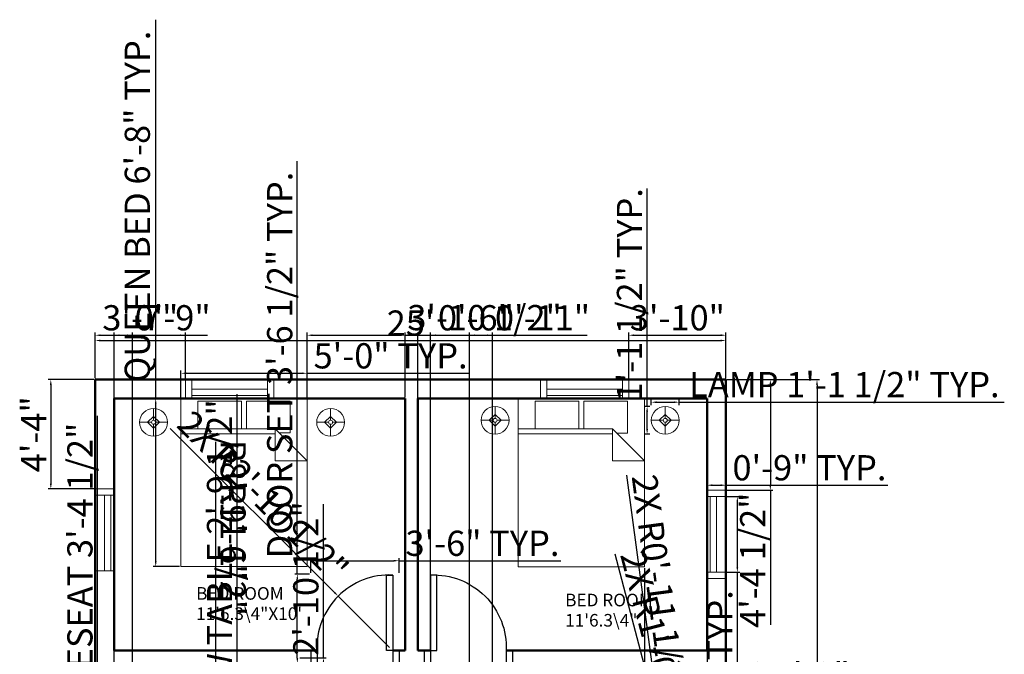
# Model space of a CAD drawing. Units: inches. Extents: x 3705 to 4206, y -1241 to -584.
# Tile 3 of 3: x 3738 to 4206, y -886 to -584. Entities that reach past the tile are written whole.
import ezdxf

# ---------------------------------------------------------------- set-up
doc = ezdxf.new("R2010")
doc.units = ezdxf.units.IN
for name, color, linetype, lineweight in [('A-ANNO-DIMS', 2, 'Continuous', 18), ('A-AREA-IDEN', 7, 'Continuous', 25), ('A-DOOR', 3, 'Continuous', 25), ('A-FURN', 8, 'Continuous', 18), ('A-GLAZ', 4, 'Continuous', 18), ('A-WALL', 7, 'Continuous', 50)]:
    doc.layers.add(name, color=color, linetype=linetype, lineweight=lineweight)
doc.styles.get("Standard").update_dxf_attribs({"font": 'arial.ttf'})
doc.dimstyles.new('ISO-25', dxfattribs={"dimtxt": 12, "dimasz": 2.5, "dimexe": 1.25, "dimexo": 0.625, "dimtad": 1, "dimdec": 1, "dimlunit": 3, "dimtxsty": 'Standard', "dimcen": 2.5, "dimadec": 0, "dimazin": 0, "dimtfac": 1, "dimtdec": 1, "dimtmove": 0, "dimatfit": 3, "dimfxl": 1, "dimarcsym": 0})

# ---------------------------------------------------------------- blocks, each defined once
blk = doc.blocks.new('Bed - Queen')
for p, q in [((0, -80.00003), (0, 0)), ((0, 0), (59.99999, 0)), ((59.99999, 0), (59.99999, -80.00003)), ((7.99999, -1.2), (28.79998, -1.2)), ((7.99999, -14.4), (7.99999, -1.2)), ((28.79998, -1.2), (28.79998, -14.4)), ((31.19999, -1.2), (51.99999, -1.2)), ((31.19999, -14.4), (31.19999, -1.2)), ((51.99999, -1.2), (51.99999, -16.4)), ((0, -14.4), (44.8, -14.4)), ((44.8, -16.8), (0, -16.8)), ((59.99999, -29.6), (44.8, -14.4)), ((44.8, -14.4), (44.8, -29.6)), ((51.99999, -16.4), (46.79936, -16.4)), ((44.8, -29.6), (59.99999, -29.6)), ((59.99999, -80.00003), (0, -80.00003))]:
    blk.add_line(p, q)
blk = doc.blocks.new('Lamp - Table')
for p, q in [((0, 7), (0, 1)), ((-1, 0), (-7, 0)), ((0, 3), (-3, 0)), ((-3, 0), (0, -3)), ((3, 0), (0, 3)), ((0, -3), (3, 0)), ((1, 0), (7, 0)), ((0, -1), (0, -7))]:
    blk.add_line(p, q)
for radius in [7, 1]:
    blk.add_circle((0, 0), radius)
blk = doc.blocks.new('*D11')
at = {"layer": 'A-ANNO-DIMS', "color": 0, "lineweight": -2, "transparency": 16777216}
for p, q in [((3774.08, -755.12), (3774.08, -735.92)), ((3776.58, -737.17), (4071.58, -737.17)), ((4074.08, -755.12), (4074.08, -735.92))]:
    blk.add_line(p, q, dxfattribs=at)
at = {"layer": 'A-ANNO-DIMS', "color": 0, "transparency": 16777216}
for points in [[(3776.58, -736.75), (3776.58, -737.58), (3774.08, -737.17)], [(4071.58, -736.75), (4071.58, -737.58), (4074.08, -737.17)]]:
    blk.add_solid(points, dxfattribs=at)
at = {"layer": 'Defpoints', "color": 0, "transparency": 16777216}
for p in [(4074.08, -737.17), (3774.08, -755.75), (4074.08, -755.75)]:
    blk.add_point(p, dxfattribs=at)
at = {"layer": 'A-ANNO-DIMS', "color": 0, "transparency": 16777216, "insert": (3924.08, -730.42), "char_height": 12, "attachment_point": 5}
blk.add_mtext("25'", dxfattribs=at)
blk = doc.blocks.new('*D12')
at = {"layer": 'A-ANNO-DIMS', "color": 0, "lineweight": -2, "transparency": 16777216}
for p, q in [((4074.7, -755.75), (4118.62, -755.75)), ((4117.37, -758.25), (4117.37, -1137.25)), ((4074.7, -1139.75), (4118.62, -1139.75))]:
    blk.add_line(p, q, dxfattribs=at)
at = {"layer": 'A-ANNO-DIMS', "color": 0, "transparency": 16777216}
for points in [[(4116.95, -758.25), (4117.78, -758.25), (4117.37, -755.75)], [(4116.95, -1137.25), (4117.78, -1137.25), (4117.37, -1139.75)]]:
    blk.add_solid(points, dxfattribs=at)
at = {"layer": 'Defpoints', "color": 0, "transparency": 16777216}
for p in [(4074.08, -755.75), (4074.08, -1139.75), (4117.37, -1139.75)]:
    blk.add_point(p, dxfattribs=at)
at = {"layer": 'A-ANNO-DIMS', "color": 0, "transparency": 16777216, "insert": (4110.61, -947.75), "char_height": 12, "attachment_point": 5, "rotation": 90}
blk.add_mtext("32'", dxfattribs=at)
blk = doc.blocks.new('DOOR-SINGLE-36IN')
for p, q in [((0, 6), (0, 0)), ((3, 6), (3, 0)), ((39, 6), (39, 0)), ((42, 6), (42, 0))]:
    blk.add_line(p, q)
blk.add_lwpolyline([(39, 6), (36, 6), (36, 42), (39, 42)], close=True)
blk.add_arc((37.5, 7.5), 34.53, 87.5104, 182.4896)
blk = doc.blocks.new('WIN-SASH-36IN')
for p, q in [((0, 9), (0, 0)), ((36, 0), (36, 9)), ((0, 4.5), (36, 4.5)), ((0, 1.5), (36, 1.5)), ((0, 1.5), (36, 1.5))]:
    blk.add_line(p, q)
blk = doc.blocks.new('*D15')
at = {"layer": 'A-ANNO-DIMS', "color": 0, "lineweight": -2, "transparency": 16777216}
for p, q in [((4074.7, -811.42), (4080.73, -811.42)), ((4079.48, -813.92), (4079.48, -844.92)), ((4074.7, -847.42), (4080.73, -847.42)), ((4079.48, -847.42), (4079.48, -1052.78))]:
    blk.add_line(p, q, dxfattribs=at)
at = {"layer": 'A-ANNO-DIMS', "color": 0, "transparency": 16777216}
for points in [[(4079.06, -813.92), (4079.9, -813.92), (4079.48, -811.42)], [(4079.06, -844.92), (4079.9, -844.92), (4079.48, -847.42)]]:
    blk.add_solid(points, dxfattribs=at)
at = {"layer": 'Defpoints', "color": 0, "transparency": 16777216}
for p in [(4074.08, -811.42), (4074.08, -847.42), (4079.48, -847.42)]:
    blk.add_point(p, dxfattribs=at)
at = {"layer": 'A-ANNO-DIMS', "color": 0, "transparency": 16777216, "insert": (4072.64, -951.35), "char_height": 12, "attachment_point": 5, "rotation": 90}
blk.add_mtext('SASH WINDOW 3\'-0" TYP.', dxfattribs=at)
blk = doc.blocks.new('*D16')
at = {"layer": 'A-ANNO-DIMS', "color": 0, "lineweight": -2, "transparency": 16777216}
for p, q in [((4065.08, -810.8), (4065.08, -804.77)), ((4074.08, -810.8), (4074.08, -804.77)), ((4067.58, -806.02), (4071.58, -806.02)), ((4074.08, -806.02), (4150.98, -806.02))]:
    blk.add_line(p, q, dxfattribs=at)
at = {"layer": 'A-ANNO-DIMS', "color": 0, "transparency": 16777216}
for points in [[(4067.58, -805.6), (4067.58, -806.44), (4065.08, -806.02)], [(4071.58, -805.6), (4071.58, -806.44), (4074.08, -806.02)]]:
    blk.add_solid(points, dxfattribs=at)
at = {"layer": 'Defpoints', "color": 0, "transparency": 16777216}
for p in [(4074.08, -806.02), (4065.08, -811.42), (4074.08, -811.42)]:
    blk.add_point(p, dxfattribs=at)
at = {"layer": 'A-ANNO-DIMS', "color": 0, "transparency": 16777216, "insert": (4113.78, -799.27), "char_height": 12, "attachment_point": 5}
blk.add_mtext('0\'-9" TYP.', dxfattribs=at)
blk = doc.blocks.new('*D17')
at = {"layer": 'A-ANNO-DIMS', "color": 0, "lineweight": -2, "transparency": 16777216}
for p, q in [((3802.87, -764.75), (3802.87, -584.48)), ((3814.24, -764.75), (3801.62, -764.75)), ((3802.87, -842.25), (3802.87, -767.25)), ((3814.24, -844.75), (3801.62, -844.75))]:
    blk.add_line(p, q, dxfattribs=at)
at = {"layer": 'A-ANNO-DIMS', "color": 0, "transparency": 16777216}
for points in [[(3802.45, -767.25), (3803.28, -767.25), (3802.87, -764.75)], [(3802.45, -842.25), (3803.28, -842.25), (3802.87, -844.75)]]:
    blk.add_solid(points, dxfattribs=at)
at = {"layer": 'Defpoints', "color": 0, "transparency": 16777216}
for p in [(3802.87, -764.75), (3814.87, -764.75), (3814.87, -844.75)]:
    blk.add_point(p, dxfattribs=at)
at = {"layer": 'A-ANNO-DIMS', "color": 0, "transparency": 16777216, "insert": (3795.67, -673.36), "char_height": 12, "attachment_point": 5, "rotation": 90}
blk.add_mtext('QUEEN BED 6\'-8" TYP.', dxfattribs=at)
blk = doc.blocks.new('*D18')
at = {"layer": 'A-ANNO-DIMS', "color": 0, "lineweight": -2, "transparency": 16777216}
for p, q in [((3814.87, -764.12), (3814.87, -751.5)), ((3817.37, -752.75), (3872.37, -752.75)), ((3874.87, -764.12), (3874.87, -751.5)), ((3874.87, -752.75), (3951.76, -752.75))]:
    blk.add_line(p, q, dxfattribs=at)
at = {"layer": 'A-ANNO-DIMS', "color": 0, "transparency": 16777216}
for points in [[(3817.37, -752.33), (3817.37, -753.16), (3814.87, -752.75)], [(3872.37, -752.33), (3872.37, -753.16), (3874.87, -752.75)]]:
    blk.add_solid(points, dxfattribs=at)
at = {"layer": 'Defpoints', "color": 0, "transparency": 16777216}
for p in [(3874.87, -752.75), (3814.87, -764.75), (3874.87, -764.75)]:
    blk.add_point(p, dxfattribs=at)
at = {"layer": 'A-ANNO-DIMS', "color": 0, "transparency": 16777216, "insert": (3914.57, -746), "char_height": 12, "attachment_point": 5}
blk.add_mtext('5\'-0" TYP.', dxfattribs=at)
blk = doc.blocks.new('*D19')
at = {"layer": 'A-ANNO-DIMS', "color": 0, "lineweight": -2, "transparency": 16777216}
for p, q in [((4038.56, -767.89), (4038.56, -765.27)), ((4041.06, -766.52), (4049.32, -766.52)), ((4051.82, -767.89), (4051.82, -765.27)), ((4051.82, -766.52), (4206.45, -766.52))]:
    blk.add_line(p, q, dxfattribs=at)
at = {"layer": 'A-ANNO-DIMS', "color": 0, "transparency": 16777216}
for points in [[(4041.06, -766.11), (4041.06, -766.94), (4038.56, -766.52)], [(4049.32, -766.11), (4049.32, -766.94), (4051.82, -766.52)]]:
    blk.add_solid(points, dxfattribs=at)
at = {"layer": 'Defpoints', "color": 0, "transparency": 16777216}
for p in [(4051.82, -766.52), (4038.56, -768.51), (4051.82, -768.51)]:
    blk.add_point(p, dxfattribs=at)
at = {"layer": 'A-ANNO-DIMS', "color": 0, "transparency": 16777216, "insert": (4130.38, -759.69), "char_height": 12, "attachment_point": 5}
blk.add_mtext('LAMP 1\'-1 1/2" TYP.', dxfattribs=at)
blk = doc.blocks.new('*D20')
at = {"layer": 'A-ANNO-DIMS', "color": 0, "lineweight": -2, "transparency": 16777216}
for p, q in [((4036.57, -768.51), (4036.57, -664.78)), ((4037.94, -768.51), (4035.32, -768.51)), ((4036.57, -779.27), (4036.57, -771.01)), ((4037.94, -781.77), (4035.32, -781.77))]:
    blk.add_line(p, q, dxfattribs=at)
at = {"layer": 'A-ANNO-DIMS', "color": 0, "transparency": 16777216}
for points in [[(4036.15, -771.01), (4036.99, -771.01), (4036.57, -768.51)], [(4036.15, -779.27), (4036.99, -779.27), (4036.57, -781.77)]]:
    blk.add_solid(points, dxfattribs=at)
at = {"layer": 'Defpoints', "color": 0, "transparency": 16777216}
for p in [(4036.57, -768.51), (4038.56, -768.51), (4038.56, -781.77)]:
    blk.add_point(p, dxfattribs=at)
at = {"layer": 'A-ANNO-DIMS', "color": 0, "transparency": 16777216, "insert": (4029.74, -715.4), "char_height": 12, "attachment_point": 5, "rotation": 90}
blk.add_mtext('1\'-1 1/2" TYP.', dxfattribs=at)
blk = doc.blocks.new('*D21')
at = {"layer": 'A-ANNO-DIMS', "color": 0, "lineweight": -2, "transparency": 16777216}
for p, q in [((3870.22, -848.33), (3870.22, -651.86)), ((3875.95, -848.33), (3868.97, -848.33)), ((3870.22, -888.25), (3870.22, -850.83)), ((3875.95, -890.75), (3868.97, -890.75))]:
    blk.add_line(p, q, dxfattribs=at)
at = {"layer": 'A-ANNO-DIMS', "color": 0, "transparency": 16777216}
for points in [[(3869.8, -850.83), (3870.63, -850.83), (3870.22, -848.33)], [(3869.8, -888.25), (3870.63, -888.25), (3870.22, -890.75)]]:
    blk.add_solid(points, dxfattribs=at)
at = {"layer": 'Defpoints', "color": 0, "transparency": 16777216}
for p in [(3870.22, -848.33), (3876.58, -848.33), (3876.58, -890.75)]:
    blk.add_point(p, dxfattribs=at)
at = {"layer": 'A-ANNO-DIMS', "color": 0, "transparency": 16777216, "insert": (3863.38, -748.84), "char_height": 12, "attachment_point": 5, "rotation": 90}
blk.add_mtext('DOOR SET 3\'-6 1/2" TYP.', dxfattribs=at)
blk = doc.blocks.new('*D22')
at = {"layer": 'A-ANNO-DIMS', "color": 0, "lineweight": -2, "transparency": 16777216}
for p, q in [((3876.58, -847.7), (3876.58, -840.71)), ((3879.08, -841.96), (3916.08, -841.96)), ((3918.58, -847.7), (3918.58, -840.71)), ((3918.58, -841.96), (3995.47, -841.96))]:
    blk.add_line(p, q, dxfattribs=at)
at = {"layer": 'A-ANNO-DIMS', "color": 0, "transparency": 16777216}
for points in [[(3879.08, -841.55), (3879.08, -842.38), (3876.58, -841.96)], [(3916.08, -841.55), (3916.08, -842.38), (3918.58, -841.96)]]:
    blk.add_solid(points, dxfattribs=at)
at = {"layer": 'Defpoints', "color": 0, "transparency": 16777216}
for p in [(3918.58, -841.96), (3876.58, -848.33), (3918.58, -848.33)]:
    blk.add_point(p, dxfattribs=at)
at = {"layer": 'A-ANNO-DIMS', "color": 0, "transparency": 16777216, "insert": (3958.27, -835.21), "char_height": 12, "attachment_point": 5}
blk.add_mtext('3\'-6" TYP.', dxfattribs=at)
blk = doc.blocks.new('*D23')
at = {"layer": 'A-ANNO-DIMS', "color": 0, "lineweight": -2, "transparency": 16777216}
for p, q in [((3775.21, -929.3), (3775.21, -773.05)), ((3780.66, -929.3), (3773.96, -929.3)), ((3775.21, -967.26), (3775.21, -931.8)), ((3780.66, -969.76), (3773.96, -969.76))]:
    blk.add_line(p, q, dxfattribs=at)
at = {"layer": 'A-ANNO-DIMS', "color": 0, "transparency": 16777216}
for points in [[(3774.79, -931.8), (3775.63, -931.8), (3775.21, -929.3)], [(3774.79, -967.26), (3775.63, -967.26), (3775.21, -969.76)]]:
    blk.add_solid(points, dxfattribs=at)
at = {"layer": 'Defpoints', "color": 0, "transparency": 16777216}
for p in [(3775.21, -929.3), (3781.28, -929.3), (3781.28, -969.76)]:
    blk.add_point(p, dxfattribs=at)
at = {"layer": 'A-ANNO-DIMS', "color": 0, "transparency": 16777216, "insert": (3768.37, -849.92), "char_height": 12, "attachment_point": 5, "rotation": 90}
blk.add_mtext('LOVESEAT 3\'-4 1/2"', dxfattribs=at)
blk = doc.blocks.new('*D26')
at = {"layer": 'A-ANNO-DIMS', "color": 0, "lineweight": -2, "transparency": 16777216}
for p, q in [((3882.65, -888.24), (3882.65, -815.1)), ((3871.43, -888.24), (3883.9, -888.24)), ((3882.65, -920.21), (3882.65, -890.74)), ((3871.43, -922.71), (3883.9, -922.71))]:
    blk.add_line(p, q, dxfattribs=at)
at = {"layer": 'A-ANNO-DIMS', "color": 0, "transparency": 16777216}
for points in [[(3882.23, -890.74), (3883.07, -890.74), (3882.65, -888.24)], [(3882.23, -920.21), (3883.07, -920.21), (3882.65, -922.71)]]:
    blk.add_solid(points, dxfattribs=at)
at = {"layer": 'Defpoints', "color": 0, "transparency": 16777216}
for p in [(3870.81, -888.24), (3882.65, -888.24), (3870.81, -922.71)]:
    blk.add_point(p, dxfattribs=at)
at = {"layer": 'A-ANNO-DIMS', "color": 0, "transparency": 16777216, "insert": (3875.82, -850.42), "char_height": 12, "attachment_point": 5, "rotation": 90}
blk.add_mtext('2\'-10 1/2"', dxfattribs=at)
blk = doc.blocks.new('*D27')
at = {"layer": 'A-ANNO-DIMS', "color": 0, "lineweight": -2, "transparency": 16777216}
for p, q in [((3841.61, -926.33), (3841.61, -762.65)), ((3837.22, -926.33), (3842.86, -926.33)), ((3841.61, -957.3), (3841.61, -928.83)), ((3837.22, -959.8), (3842.86, -959.8))]:
    blk.add_line(p, q, dxfattribs=at)
at = {"layer": 'A-ANNO-DIMS', "color": 0, "transparency": 16777216}
for points in [[(3841.2, -928.83), (3842.03, -928.83), (3841.61, -926.33)], [(3841.2, -957.3), (3842.03, -957.3), (3841.61, -959.8)]]:
    blk.add_solid(points, dxfattribs=at)
at = {"layer": 'Defpoints', "color": 0, "transparency": 16777216}
for p in [(3836.59, -926.33), (3841.61, -926.33), (3836.59, -959.8)]:
    blk.add_point(p, dxfattribs=at)
at = {"layer": 'A-ANNO-DIMS', "color": 0, "transparency": 16777216, "insert": (3834.78, -843.24), "char_height": 12, "attachment_point": 5, "rotation": 90}
blk.add_mtext('LOW TABLE 2\'-9 1/2"', dxfattribs=at)
blk = doc.blocks.new('*D29')
at = {"layer": 'A-ANNO-DIMS', "color": 0, "lineweight": -2, "transparency": 16777216}
for p, q in [((4032.03, -908.99), (4032.03, -903.41)), ((4065.08, -908.99), (4065.08, -903.41)), ((4034.53, -904.66), (4062.58, -904.66)), ((4065.08, -904.66), (4133.81, -904.66))]:
    blk.add_line(p, q, dxfattribs=at)
at = {"layer": 'A-ANNO-DIMS', "color": 0, "transparency": 16777216}
for points in [[(4034.53, -904.24), (4034.53, -905.07), (4032.03, -904.66)], [(4062.58, -904.24), (4062.58, -905.07), (4065.08, -904.66)]]:
    blk.add_solid(points, dxfattribs=at)
at = {"layer": 'Defpoints', "color": 0, "transparency": 16777216}
for p in [(4065.08, -904.66), (4032.03, -909.61), (4065.08, -909.61)]:
    blk.add_point(p, dxfattribs=at)
at = {"layer": 'A-ANNO-DIMS', "color": 0, "transparency": 16777216, "insert": (4100.69, -897.83), "char_height": 12, "attachment_point": 5}
blk.add_mtext('WC 2\'-9"', dxfattribs=at)
blk = doc.blocks.new('*D35')
at = {"layer": 'A-ANNO-DIMS', "color": 0, "lineweight": -2, "transparency": 16777216}
for p, q in [((3774.08, -755.12), (3774.08, -733.4)), ((3776.58, -734.65), (3814.52, -734.65)), ((3817.02, -755.12), (3817.02, -733.4))]:
    blk.add_line(p, q, dxfattribs=at)
at = {"layer": 'A-ANNO-DIMS', "color": 0, "transparency": 16777216}
for points in [[(3776.58, -734.23), (3776.58, -735.06), (3774.08, -734.65)], [(3814.52, -734.23), (3814.52, -735.06), (3817.02, -734.65)]]:
    blk.add_solid(points, dxfattribs=at)
at = {"layer": 'Defpoints', "color": 0, "transparency": 16777216}
for p in [(3817.02, -734.65), (3774.08, -755.75), (3817.02, -755.75)]:
    blk.add_point(p, dxfattribs=at)
at = {"layer": 'A-ANNO-DIMS', "color": 0, "transparency": 16777216, "insert": (3795.55, -727.89), "char_height": 12, "attachment_point": 5}
blk.add_mtext('3\'-7"', dxfattribs=at)
blk = doc.blocks.new('*D36')
at = {"layer": 'A-ANNO-DIMS', "color": 0, "lineweight": -2, "transparency": 16777216}
for p, q in [((4027.86, -755.12), (4027.86, -733.4)), ((4030.36, -734.65), (4071.58, -734.65)), ((4074.08, -755.12), (4074.08, -733.4))]:
    blk.add_line(p, q, dxfattribs=at)
at = {"layer": 'A-ANNO-DIMS', "color": 0, "transparency": 16777216}
for points in [[(4030.36, -734.23), (4030.36, -735.06), (4027.86, -734.65)], [(4071.58, -734.23), (4071.58, -735.06), (4074.08, -734.65)]]:
    blk.add_solid(points, dxfattribs=at)
at = {"layer": 'Defpoints', "color": 0, "transparency": 16777216}
for p in [(4074.08, -734.65), (4027.86, -755.75), (4074.08, -755.75)]:
    blk.add_point(p, dxfattribs=at)
at = {"layer": 'A-ANNO-DIMS', "color": 0, "transparency": 16777216, "insert": (4050.97, -727.89), "char_height": 12, "attachment_point": 5}
blk.add_mtext('3\'-10"', dxfattribs=at)
blk = doc.blocks.new('*D37')
at = {"layer": 'A-ANNO-DIMS', "color": 0, "lineweight": -2, "transparency": 16777216}
for p, q in [((3773.45, -755.75), (3751.73, -755.75)), ((3752.98, -758.25), (3752.98, -805.28)), ((3773.45, -807.78), (3751.73, -807.78))]:
    blk.add_line(p, q, dxfattribs=at)
at = {"layer": 'A-ANNO-DIMS', "color": 0, "transparency": 16777216}
for points in [[(3752.56, -758.25), (3753.4, -758.25), (3752.98, -755.75)], [(3752.56, -805.28), (3753.4, -805.28), (3752.98, -807.78)]]:
    blk.add_solid(points, dxfattribs=at)
at = {"layer": 'Defpoints', "color": 0, "transparency": 16777216}
for p in [(3774.08, -755.75), (3752.98, -807.78), (3774.08, -807.78)]:
    blk.add_point(p, dxfattribs=at)
at = {"layer": 'A-ANNO-DIMS', "color": 0, "transparency": 16777216, "insert": (3746.35, -781.77), "char_height": 12, "attachment_point": 5, "rotation": 90}
blk.add_mtext('4\'-4"', dxfattribs=at)
blk = doc.blocks.new('*D38')
at = {"layer": 'A-ANNO-DIMS', "color": 0, "lineweight": -2, "transparency": 16777216}
for p, q in [((4074.7, -755.75), (4096.43, -755.75)), ((4095.18, -758.25), (4095.18, -805.92)), ((4074.7, -808.42), (4096.43, -808.42)), ((4095.18, -808.42), (4095.18, -872.51))]:
    blk.add_line(p, q, dxfattribs=at)
at = {"layer": 'A-ANNO-DIMS', "color": 0, "transparency": 16777216}
for points in [[(4094.76, -758.25), (4095.6, -758.25), (4095.18, -755.75)], [(4094.76, -805.92), (4095.6, -805.92), (4095.18, -808.42)]]:
    blk.add_solid(points, dxfattribs=at)
at = {"layer": 'Defpoints', "color": 0, "transparency": 16777216}
for p in [(4074.08, -755.75), (4074.08, -808.42), (4095.18, -808.42)]:
    blk.add_point(p, dxfattribs=at)
at = {"layer": 'A-ANNO-DIMS', "color": 0, "transparency": 16777216, "insert": (4088.35, -841.72), "char_height": 12, "attachment_point": 5, "rotation": 90}
blk.add_mtext('4\'-4 1/2"', dxfattribs=at)
blk = doc.blocks.new('*D52')
at = {"layer": 'A-ANNO-DIMS', "color": 0, "lineweight": -2, "transparency": 16777216}
for p, q in [((3925.08, -734.65), (3922.58, -734.65)), ((3927.58, -884.12), (3927.58, -733.4)), ((3927.58, -734.65), (3933.58, -734.65)), ((3933.58, -884.12), (3933.58, -733.4)), ((3936.08, -734.65), (3971.73, -734.65))]:
    blk.add_line(p, q, dxfattribs=at)
at = {"layer": 'A-ANNO-DIMS', "color": 0, "transparency": 16777216}
for points in [[(3925.08, -734.23), (3925.08, -735.06), (3927.58, -734.65)], [(3936.08, -734.23), (3936.08, -735.06), (3933.58, -734.65)]]:
    blk.add_solid(points, dxfattribs=at)
at = {"layer": 'Defpoints', "color": 0, "transparency": 16777216}
for p in [(3933.58, -734.65), (3927.58, -884.75), (3933.58, -884.75)]:
    blk.add_point(p, dxfattribs=at)
at = {"layer": 'A-ANNO-DIMS', "color": 0, "transparency": 16777216, "insert": (3955.15, -727.9), "char_height": 12, "attachment_point": 5}
blk.add_mtext('0\'-6"', dxfattribs=at)
blk = doc.blocks.new('*D53')
at = {"layer": 'A-ANNO-DIMS', "color": 0, "lineweight": -2, "transparency": 16777216}
for p, q in [((3952.08, -1130.12), (3952.08, -733.4)), ((3954.58, -734.65), (3960.58, -734.65)), ((3963.08, -1130.12), (3963.08, -733.4)), ((3963.08, -734.65), (4008.05, -734.65))]:
    blk.add_line(p, q, dxfattribs=at)
at = {"layer": 'A-ANNO-DIMS', "color": 0, "transparency": 16777216}
for points in [[(3954.58, -734.23), (3954.58, -735.06), (3952.08, -734.65)], [(3960.58, -734.23), (3960.58, -735.06), (3963.08, -734.65)]]:
    blk.add_solid(points, dxfattribs=at)
at = {"layer": 'Defpoints', "color": 0, "transparency": 16777216}
for p in [(3963.08, -734.65), (3952.08, -1130.75), (3963.08, -1130.75)]:
    blk.add_point(p, dxfattribs=at)
at = {"layer": 'A-ANNO-DIMS', "color": 0, "transparency": 16777216, "insert": (3986.82, -727.9), "char_height": 12, "attachment_point": 5}
blk.add_mtext('0\'-11"', dxfattribs=at)
blk = doc.blocks.new('*D54')
at = {"layer": 'A-ANNO-DIMS', "color": 0, "lineweight": -2, "transparency": 16777216}
for p, q in [((3874.87, -764.12), (3874.87, -733.4)), ((3877.37, -734.65), (3919.08, -734.65)), ((3921.58, -764.12), (3921.58, -733.4)), ((3921.58, -734.65), (3994.51, -734.65))]:
    blk.add_line(p, q, dxfattribs=at)
at = {"layer": 'A-ANNO-DIMS', "color": 0, "transparency": 16777216}
for points in [[(3877.37, -734.23), (3877.37, -735.06), (3874.87, -734.65)], [(3919.08, -734.23), (3919.08, -735.06), (3921.58, -734.65)]]:
    blk.add_solid(points, dxfattribs=at)
at = {"layer": 'Defpoints', "color": 0, "transparency": 16777216}
for p in [(3921.58, -734.65), (3874.87, -764.75), (3921.58, -764.75)]:
    blk.add_point(p, dxfattribs=at)
at = {"layer": 'A-ANNO-DIMS', "color": 0, "transparency": 16777216, "insert": (3959.29, -727.81), "char_height": 12, "attachment_point": 5}
blk.add_mtext('3\'-10 1/2"', dxfattribs=at)
blk = doc.blocks.new('*D55')
at = {"layer": 'A-ANNO-DIMS', "color": 0, "lineweight": -2, "transparency": 16777216}
for p, q in [((4035.32, -845.43), (4035.32, -1162.1)), ((4065.08, -851.05), (4065.08, -1162.1)), ((4037.82, -1160.85), (4062.58, -1160.85)), ((4065.08, -1160.85), (4100.93, -1160.85))]:
    blk.add_line(p, q, dxfattribs=at)
at = {"layer": 'A-ANNO-DIMS', "color": 0, "transparency": 16777216}
for points in [[(4037.82, -1160.43), (4037.82, -1161.26), (4035.32, -1160.85)], [(4062.58, -1160.43), (4062.58, -1161.26), (4065.08, -1160.85)]]:
    blk.add_solid(points, dxfattribs=at)
at = {"layer": 'Defpoints', "color": 0, "transparency": 16777216}
for p in [(4035.32, -844.8), (4065.08, -850.42), (4065.08, -1160.85)]:
    blk.add_point(p, dxfattribs=at)
at = {"layer": 'A-ANNO-DIMS', "color": 0, "transparency": 16777216, "insert": (4084.26, -1154.1), "char_height": 12, "attachment_point": 5}
blk.add_mtext('2\'-6"', dxfattribs=at)
blk = doc.blocks.new('*D56')
at = {"layer": 'A-ANNO-DIMS', "color": 0, "lineweight": -2, "transparency": 16777216}
for p, q in [((3783.08, -890.12), (3783.08, -733.4)), ((3785.58, -734.65), (3789.35, -734.65)), ((3791.85, -897.64), (3791.85, -733.4)), ((3791.85, -734.65), (3827.5, -734.65))]:
    blk.add_line(p, q, dxfattribs=at)
at = {"layer": 'A-ANNO-DIMS', "color": 0, "transparency": 16777216}
for points in [[(3785.58, -734.23), (3785.58, -735.06), (3783.08, -734.65)], [(3789.35, -734.23), (3789.35, -735.06), (3791.85, -734.65)]]:
    blk.add_solid(points, dxfattribs=at)
at = {"layer": 'Defpoints', "color": 0, "transparency": 16777216}
for p in [(3791.85, -734.65), (3783.08, -890.75), (3791.85, -898.27)]:
    blk.add_point(p, dxfattribs=at)
at = {"layer": 'A-ANNO-DIMS', "color": 0, "transparency": 16777216, "insert": (3810.93, -727.9), "char_height": 12, "attachment_point": 5}
blk.add_mtext('0\'-9"', dxfattribs=at)
blk = doc.blocks.new('*D60')
at = {"layer": 'A-ANNO-DIMS', "color": 0, "lineweight": -2, "transparency": 16777216}
for p, q in [((3831.33, -805.72), (3831.33, -893.89)), ((3831.33, -1010.31), (3831.33, -896.39))]:
    blk.add_line(p, q, dxfattribs=at)
at = {"layer": 'A-ANNO-DIMS', "color": 0, "transparency": 16777216}
blk.add_solid([(3831.75, -893.89), (3830.91, -893.89), (3831.33, -896.39)], dxfattribs=at)
at = {"layer": 'Defpoints', "color": 0, "transparency": 16777216}
for p in [(3831.33, -896.39), (3831.33, -1010.31)]:
    blk.add_point(p, dxfattribs=at)
at = {"layer": 'A-ANNO-DIMS', "color": 0, "transparency": 16777216, "insert": (3838.08, -828.04), "char_height": 12, "attachment_point": 5, "rotation": 270.0001}
blk.add_mtext('R9\'-6"', dxfattribs=at)
blk = doc.blocks.new('*D61')
at = {"layer": 'A-ANNO-DIMS', "color": 0, "lineweight": -2, "transparency": 16777216}
for p, q in [((3831.33, -785.35), (3831.33, -888.25)), ((3831.33, -998.14), (3831.33, -890.75))]:
    blk.add_line(p, q, dxfattribs=at)
at = {"layer": 'A-ANNO-DIMS', "color": 0, "transparency": 16777216}
blk.add_solid([(3831.75, -888.25), (3830.91, -888.25), (3831.33, -890.75)], dxfattribs=at)
at = {"layer": 'Defpoints', "color": 0, "transparency": 16777216}
for p in [(3831.33, -890.75), (3831.33, -998.14)]:
    blk.add_point(p, dxfattribs=at)
at = {"layer": 'A-ANNO-DIMS', "color": 0, "transparency": 16777216, "insert": (3838.16, -826.31), "char_height": 12, "attachment_point": 5, "rotation": 270.0001}
blk.add_mtext('R8\'-11 1/2"', dxfattribs=at)
blk = doc.blocks.new('*D65')
at = {"layer": 'A-ANNO-DIMS', "color": 0, "lineweight": -2, "transparency": 16777216}
for p, q in [((3809.82, -778.99), (3887.89, -857.06)), ((3914.08, -883.25), (3889.66, -858.83))]:
    blk.add_line(p, q, dxfattribs=at)
at = {"layer": 'A-ANNO-DIMS', "color": 0, "transparency": 16777216}
blk.add_solid([(3888.19, -856.77), (3887.6, -857.36), (3889.66, -858.83)], dxfattribs=at)
at = {"layer": 'Defpoints', "color": 0, "transparency": 16777216}
for p in [(3889.66, -858.83), (3914.08, -883.25)]:
    blk.add_point(p, dxfattribs=at)
at = {"layer": 'A-ANNO-DIMS', "color": 0, "transparency": 16777216, "insert": (3852.8, -812.31), "char_height": 12, "attachment_point": 5, "rotation": 315}
blk.add_mtext('2X R2\'-10 1/2"', dxfattribs=at)
blk = doc.blocks.new('*D66')
at = {"layer": 'A-ANNO-DIMS', "color": 0, "lineweight": -2, "transparency": 16777216}
for p, q in [((4021.19, -838.72), (4039.77, -909.45)), ((4043.5, -923.63), (4040.41, -911.86))]:
    blk.add_line(p, q, dxfattribs=at)
at = {"layer": 'A-ANNO-DIMS', "color": 0, "transparency": 16777216}
blk.add_solid([(4040.17, -909.34), (4039.37, -909.55), (4040.41, -911.86)], dxfattribs=at)
at = {"layer": 'Defpoints', "color": 0, "transparency": 16777216}
for p in [(4040.41, -911.86), (4043.5, -923.63)]:
    blk.add_point(p, dxfattribs=at)
at = {"layer": 'A-ANNO-DIMS', "color": 0, "transparency": 16777216, "insert": (4036.7, -871.16), "char_height": 12, "attachment_point": 5, "rotation": 284.7176}
blk.add_mtext('2X R1\'-0"', dxfattribs=at)
blk = doc.blocks.new('*D67')
at = {"layer": 'A-ANNO-DIMS', "color": 0, "lineweight": -2, "transparency": 16777216}
for p, q in [((4026.71, -801.19), (4041.42, -910.61)), ((4043.26, -924.31), (4041.75, -913.09))]:
    blk.add_line(p, q, dxfattribs=at)
at = {"layer": 'A-ANNO-DIMS', "color": 0, "transparency": 16777216}
blk.add_solid([(4041.83, -910.55), (4041.01, -910.66), (4041.75, -913.09)], dxfattribs=at)
at = {"layer": 'Defpoints', "color": 0, "transparency": 16777216}
for p in [(4041.75, -913.09), (4043.26, -924.31)]:
    blk.add_point(p, dxfattribs=at)
at = {"layer": 'A-ANNO-DIMS', "color": 0, "transparency": 16777216, "insert": (4040.66, -853.75), "char_height": 12, "attachment_point": 5, "rotation": 277.6579}
blk.add_mtext('2X R0\'-11 1/2"', dxfattribs=at)

msp = doc.modelspace()

# ---------------------------------------------------------------- linework, layer by layer
at = {"layer": 'A-GLAZ'}
for p, q in [((3817.02, -755.75), (3817.02, -764.75)), ((3856.02, -755.75), (3820.02, -755.75)), ((3859.02, -764.75), (3859.02, -755.75)), ((3985.86, -755.75), (3985.86, -764.75)), ((4027.86, -764.75), (4027.86, -755.75)), ((3820.02, -764.75), (3856.02, -764.75)), ((3783.08, -807.78), (3774.08, -807.78)), ((4074.08, -808.42), (4065.08, -808.42)), ((4065.08, -850.42), (4074.08, -850.42))]:
    msp.add_line(p, q, dxfattribs=at)
at = {"layer": 'A-WALL'}
for p, q in [((3783.08, -764.75), (3783.08, -884.75)), ((3921.58, -764.75), (3783.08, -764.75)), ((3921.58, -764.75), (3921.58, -884.75)), ((4065.08, -764.75), (3927.58, -764.75)), ((3927.58, -764.75), (3927.58, -884.75)), ((4065.08, -884.75), (4065.08, -764.75)), ((3879.58, -884.75), (3783.08, -884.75)), ((3921.58, -884.75), (3915.58, -884.75)), ((3933.58, -884.75), (3927.58, -884.75)), ((4065.08, -884.75), (3969.58, -884.75))]:
    msp.add_line(p, q, dxfattribs=at)
msp.add_lwpolyline([(3909.08, -1139.75), (4074.08, -1139.75), (4074.08, -755.75), (3774.08, -755.75), (3774.08, -1139.75), (3789.08, -1139.75)], dxfattribs=at)

# ---------------------------------------------------------------- block references
at = {"layer": 'A-DOOR'}
msp.add_blockref('DOOR-SINGLE-36IN', (3876.58, -890.75), dxfattribs=at)
at = {"layer": 'A-DOOR', "extrusion": (0, 0, -1), "zscale": -1}
msp.add_blockref('DOOR-SINGLE-36IN', (-3972.58, -890.75), dxfattribs=at)
at = {"layer": 'A-FURN'}
for p in [(3814.87, -764.75), (3975.32, -764.8)]:
    msp.add_blockref('Bed - Queen', p, dxfattribs=at)
at = {"layer": 'A-FURN', "xscale": 0.946953533406538, "yscale": 0.946953533406538, "zscale": 0.946953533406538}
for p in [(3801.84, -776.09), (3886.05, -776.09), (3964.27, -775.14), (4045.19, -775.14)]:
    msp.add_blockref('Lamp - Table', p, dxfattribs=at)
at = {"layer": 'A-GLAZ'}
for p in [(3820.02, -764.75), (3988.86, -764.75)]:
    msp.add_blockref('WIN-SASH-36IN', p, dxfattribs=at)
for p, rotation in [((3783.08, -846.78), 89.9999999999985), ((4065.08, -811.42), 269.9999999999986)]:
    msp.add_blockref('WIN-SASH-36IN', p, dxfattribs=dict(at, rotation=rotation))

# ---------------------------------------------------------------- texts
at = {"layer": 'A-AREA-IDEN'}
for s, p in [('BED ROOM', (3822.08, -860.51)), ('BED ROOM', (3997.6, -863.66)), ('11\'6.3\\4"X10\'', (3822.08, -870.15)), ('11\'6.3\\4"', (3997.6, -873.3))]:
    msp.add_text(s, height=6, dxfattribs=at).set_placement(p)

# ---------------------------------------------------------------- dimensions: what is measured, and where the dimension line sits
at = {"layer": 'A-ANNO-DIMS'}
for base, p1, p2, angle, text, picture, middle in [((3802.87, -764.75), (3814.87, -844.75), (3814.87, -764.75), 90, 'QUEEN BED <> TYP.', '*D17', (3795.67, -673.36)), ((3870.22, -848.33), (3876.58, -890.75), (3876.58, -848.33), 90, 'DOOR SET <> TYP.', '*D21', (3863.38, -748.84)), ((4036.57, -768.51), (4038.56, -781.77), (4038.56, -768.51), 90, '<> TYP.', '*D20', (4029.74, -715.4)), ((3841.61, -926.33), (3836.59, -959.8), (3836.59, -926.33), 90, 'LOW TABLE <>', '*D27', (3834.78, -843.24)), ((3775.21, -929.3), (3781.28, -969.76), (3781.28, -929.3), 90, 'LOVESEAT <>', '*D23', (3768.37, -849.92)), ((4079.48, -847.42), (4074.08, -811.42), (4074.08, -847.42), 270, 'SASH WINDOW <> TYP.', '*D15', (4072.64, -951.35))]:
    dim = msp.add_linear_dim(base=base, p1=p1, p2=p2, angle=angle, text=text, dimstyle='ISO-25', override={"dimdec": 1, "dimlfac": 1, "dimrnd": 0, "dimzin": 1, "dimdsep": 46, "dimlunit": 4, "dimfrac": 2}, dxfattribs=at)
    dim.commit()
    dim.dimension.update_dxf_attribs({"geometry": picture, "text_midpoint": middle})
for base, p1, p2, override, picture, middle in [((3921.58, -734.65), (3874.87, -764.75), (3921.58, -764.75), {"dimdec": 1, "dimlfac": 1, "dimrnd": 0, "dimzin": 1, "dimdsep": 46, "dimlunit": 4, "dimfrac": 2}, '*D54', (3959.29, -727.81)), ((3817.02, -734.65), (3774.08, -755.75), (3817.02, -755.75), {"dimdec": 1, "dimlfac": 1, "dimrnd": 0, "dimzin": 1, "dimdsep": 46, "dimlunit": 4, "dimfrac": 2}, '*D35', (3795.55, -727.89)), ((3791.85, -734.65), (3783.08, -890.75), (3791.85, -898.27), {"dimdec": 1, "dimlfac": 1, "dimrnd": 0, "dimzin": 1, "dimdsep": 46, "dimlunit": 4, "dimfrac": 2}, '*D56', (3810.93, -727.9)), ((3933.58, -734.65), (3927.58, -884.75), (3933.58, -884.75), {"dimdec": 1, "dimlfac": 1, "dimrnd": 0, "dimzin": 1, "dimdsep": 46, "dimlunit": 4, "dimfrac": 2}, '*D52', (3955.15, -727.9)), ((3963.08, -734.65), (3952.08, -1130.75), (3963.08, -1130.75), {"dimdec": 1, "dimlfac": 1, "dimrnd": 0, "dimzin": 1, "dimdsep": 46, "dimlunit": 4, "dimfrac": 2}, '*D53', (3986.82, -727.9)), ((4074.08, -734.65), (4027.86, -755.75), (4074.08, -755.75), {"dimdec": 1, "dimlfac": 1, "dimrnd": 0, "dimzin": 1, "dimdsep": 46, "dimlunit": 4, "dimfrac": 2}, '*D36', (4050.97, -727.89)), ((4074.08, -737.17), (3774.08, -755.75), (4074.08, -755.75), {"dimclrd": 0, "dimclre": 0, "dimclrt": 0}, '*D11', (3924.08, -730.42)), ((4065.08, -1160.85), (4035.32, -844.8), (4065.08, -850.42), {"dimdec": 1, "dimlfac": 1, "dimrnd": 0, "dimzin": 1, "dimdsep": 46, "dimlunit": 4, "dimfrac": 2}, '*D55', (4084.26, -1154.1))]:
    dim = msp.add_linear_dim(base=base, p1=p1, p2=p2, dimstyle='ISO-25', override=override, dxfattribs=at)
    dim.commit()
    dim.dimension.update_dxf_attribs({"geometry": picture, "text_midpoint": middle})
for base, p1, p2, text, picture, middle in [((4051.82, -766.52), (4038.56, -768.51), (4051.82, -768.51), 'LAMP <> TYP.', '*D19', (4130.38, -759.69)), ((3874.87, -752.75), (3814.87, -764.75), (3874.87, -764.75), '<> TYP.', '*D18', (3914.57, -746)), ((4074.08, -806.02), (4065.08, -811.42), (4074.08, -811.42), '<> TYP.', '*D16', (4113.78, -799.27)), ((3918.58, -841.96), (3876.58, -848.33), (3918.58, -848.33), '<> TYP.', '*D22', (3958.27, -835.21)), ((4065.0791, -904.6575), (4032.0329, -909.6144), (4065.0791, -909.6144), 'WC <>', '*D29', (4100.6926, -897.8278))]:
    dim = msp.add_linear_dim(base=base, p1=p1, p2=p2, text=text, dimstyle='ISO-25', override={"dimdec": 1, "dimlfac": 1, "dimrnd": 0, "dimzin": 1, "dimdsep": 46, "dimlunit": 4, "dimfrac": 2}, dxfattribs=at)
    dim.commit()
    dim.dimension.update_dxf_attribs({"geometry": picture, "text_midpoint": middle})
for base, p1, p2, override, picture, middle in [((3752.98, -807.78), (3774.08, -755.75), (3774.08, -807.78), {"dimdec": 1, "dimlfac": 1, "dimrnd": 0, "dimzin": 1, "dimdsep": 46, "dimlunit": 4, "dimfrac": 2}, '*D37', (3746.35, -781.77)), ((4095.18, -808.42), (4074.08, -755.75), (4074.08, -808.42), {"dimdec": 1, "dimlfac": 1, "dimrnd": 0, "dimzin": 1, "dimdsep": 46, "dimlunit": 4, "dimfrac": 2}, '*D38', (4088.35, -841.72)), ((4117.37, -1139.75), (4074.08, -755.75), (4074.08, -1139.75), {"dimclrd": 0, "dimclre": 0, "dimclrt": 0}, '*D12', (4110.61, -947.75)), ((3882.65, -888.24), (3870.81, -922.71), (3870.81, -888.24), {"dimdec": 1, "dimlfac": 1, "dimrnd": 0, "dimzin": 1, "dimdsep": 46, "dimlunit": 4, "dimfrac": 2}, '*D26', (3875.82, -850.42))]:
    dim = msp.add_linear_dim(base=base, p1=p1, p2=p2, angle=90, dimstyle='ISO-25', override=override, dxfattribs=at)
    dim.commit()
    dim.dimension.update_dxf_attribs({"geometry": picture, "text_midpoint": middle})
for center, mpoint, picture, middle in [((3914.08, -883.25), (3889.66, -858.83), '*D65', (3852.8, -812.31)), ((4043.26, -924.31), (4041.75, -913.09), '*D67', (4040.66, -853.75)), ((4043.5, -923.63), (4040.41, -911.86), '*D66', (4036.7, -871.16))]:
    dim = msp.add_radius_dim(center=center, mpoint=mpoint, text='2X <>', dimstyle='ISO-25', override={"dimdec": 1, "dimlfac": 1, "dimrnd": 0, "dimzin": 1, "dimdsep": 46, "dimlunit": 4, "dimfrac": 2}, dxfattribs=at)
    dim.commit()
    dim.dimension.update_dxf_attribs({"geometry": picture, "text_midpoint": middle})
for center, mpoint, picture, middle in [((3831.33, -998.14), (3831.33, -890.75), '*D61', (3831.33, -826.31)), ((3831.33, -1010.31), (3831.33, -896.39), '*D60', (3831.33, -828.04))]:
    dim = msp.add_radius_dim(center=center, mpoint=mpoint, dimstyle='ISO-25', override={"dimdec": 1, "dimlfac": 1, "dimrnd": 0, "dimzin": 1, "dimdsep": 46, "dimlunit": 4, "dimfrac": 2}, dxfattribs=at)
    dim.commit()
    dim.dimension.update_dxf_attribs({"geometry": picture, "text_midpoint": middle, "dimtype": 164})

doc.saveas('drawing.dxf')
